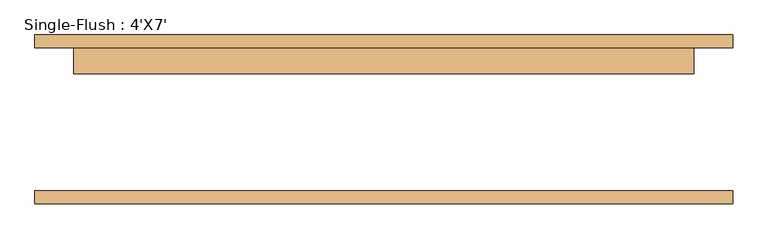
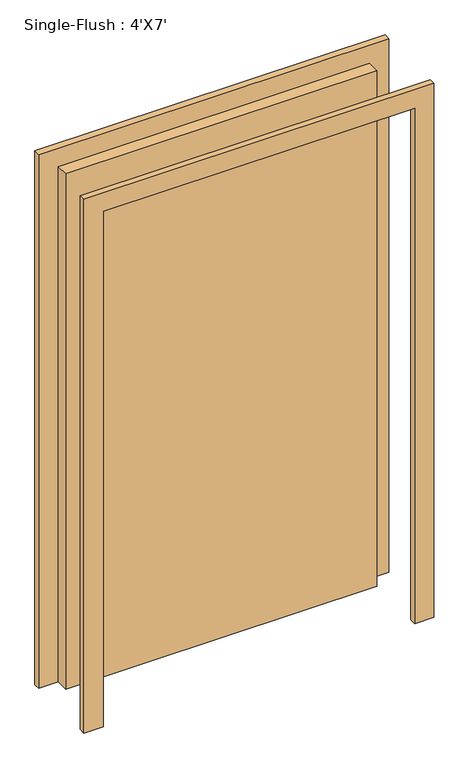
"""IFC4 building model written with IfcOpenShell, lengths in millimetres: door geometry, Single-Flush : 4'X7'."""

from ifc_helpers import new_model, si_unit, frame, origin, origin_with_axes, place, context, project, spatial, polyline, outline, extrude, source, transform, mapped, element, save


def single_flush_4_x7_4e2c9459(model_context):
    return source(origin(), model_context, "Body", "SweptSolid", [
        extrude(outline(polyline([(2209.8, -685.8), (0.0, -685.8), (0.0, -609.6), (2133.6, -609.6), (2133.6, 609.6), (0.0, 609.6), (0.0, 685.8), (2209.8, 685.8), (2209.8, -685.8)])), frame((0.0, 140.4, 0.0), z_axis=(0.0, 1.0, 0.0), x_axis=(0.0, 0.0, 1.0)), (0.0, 0.0, 1.0), 25.4),
        extrude(outline(polyline([(2209.8, 685.8), (2209.8, -685.8), (0.0, -685.8), (0.0, -609.6), (2133.6, -609.6), (2133.6, 609.6), (0.0, 609.6), (0.0, 685.8), (2209.8, 685.8)])), frame((0.0, -165.8, 0.0), z_axis=(0.0, 1.0, 0.0), x_axis=(0.0, 0.0, 1.0)), (0.0, 0.0, 1.0), 25.4),
        extrude(outline(polyline([(609.6, 89.6), (-609.6, 89.6), (-609.6, 140.4), (609.6, 140.4), (609.6, 89.6)])), origin_with_axes(), (0.0, 0.0, 1.0), 2133.6),
    ])


if __name__ == "__main__":
    model = new_model("IFC4")
    model_context = context("Model", 3, world=origin())
    ifc_project = project(units=[si_unit("LENGTHUNIT", "METRE", prefix="MILLI")], contexts=[model_context])
    site = spatial("IfcSite", under=ifc_project)
    building = spatial("IfcBuilding", under=site)
    placement = place(None, origin())
    single_flush_4_x7_shape = single_flush_4_x7_4e2c9459(model_context)
    element("IfcDoor", 1, ObjectType="Single-Flush : 4'X7'", at=placement, inside=building, context=model_context, shape_type="MappedRepresentation", body=[
        mapped(single_flush_4_x7_shape, transform((0.0, 0.0, 0.0), x_axis=(1.0, 0.0, 0.0), y_axis=(0.0, 1.0, 0.0), z_axis=(0.0, 0.0, 1.0))),
    ])
    save(model, "model.ifc")

# Revit data of these elements
# Type "Single-Flush : 4'X7'"
#   Type Mark = "11"
#   Assembly Code = "C1020"
#   Thickness = 0' - 2"
#   Height = 7' - 0"
#   Trim Projection Ext = 0' - 1"
#   Trim Projection Int = 0' - 1"
#   Trim Width = 0' - 3"
#   Width = 4' - 0"
#   Door Material = Door - Panel
#   Frame Material = Door - Frame
#   Function = (empty or 0)
#   Wall Closure = (empty or 0)
# Element 1 (IfcDoor, "Single-Flush : 4'X7'")
#   Materials on its faces: "Door - Frame", "Door - Panel"
# Materials
#   "Door - Panel": class "Wood", colour RGB 114 82 51, transparency 0
#   "Door - Frame": colour RGB 153 76 43, transparency 0
